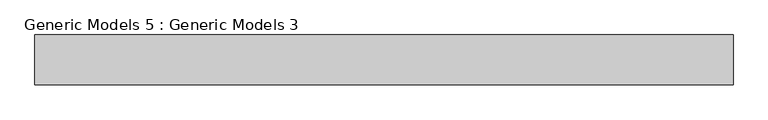
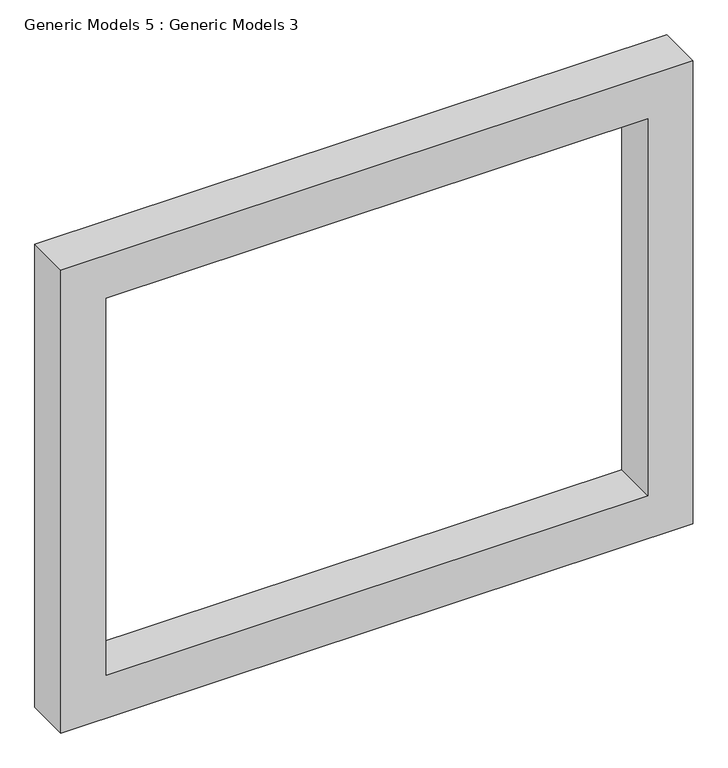
"""IFC4 building model written with IfcOpenShell, lengths in millimetres: proxy geometry, Generic Models 5 : Generic Models 3."""

from ifc_helpers import new_model, si_unit, frame, origin, place, context, project, spatial, polyline, outline, extrude, source, transform, mapped, element, save


def generic_models_5_generic_models_3_e9287e6f(model_context):
    return source(origin(), model_context, "Body", "SweptSolid", [
        extrude(outline(polyline([(5765.8, 4938.2671209), (5765.8, 2804.6671209), (4114.8, 2804.6671209), (4114.8, 4938.2671209), (5765.8, 4938.2671209)]), holes=[polyline([(5613.4, 4785.8671209), (4267.2, 4785.8671209), (4267.2, 2957.0671209), (5613.4, 2957.0671209), (5613.4, 4785.8671209)])]), frame((0.0, -2602.2776789, 0.0), z_axis=(0.0, 1.0, 0.0), x_axis=(0.0, 0.0, 1.0)), (0.0, 0.0, 1.0), 152.4),
    ])


if __name__ == "__main__":
    model = new_model("IFC4")
    model_context = context("Model", 3, world=origin())
    ifc_project = project(units=[si_unit("LENGTHUNIT", "METRE", prefix="MILLI")], contexts=[model_context])
    site = spatial("IfcSite", under=ifc_project)
    building = spatial("IfcBuilding", under=site)
    placement = place(None, origin())
    generic_models_5_generic_models_3_shape = generic_models_5_generic_models_3_e9287e6f(model_context)
    element("IfcBuildingElementProxy", 1, Name="Generic Models 5 : Generic Models 3", ObjectType="Generic Models 5 : Generic Models 3", at=placement, inside=building, context=model_context, shape_type="MappedRepresentation", body=[
        mapped(generic_models_5_generic_models_3_shape, transform((0.0, 0.0, 0.0), x_axis=(1.0, 0.0, 0.0), y_axis=(0.0, 1.0, 0.0), z_axis=(0.0, 0.0, 1.0))),
    ])
    save(model, "model.ifc")

# Revit data of these elements
# Element 1 (IfcBuildingElementProxy, "Generic Models 5 : Generic Models 3")
#   Materials on its faces: "WALNUT WOOD COLOUR 5\""
# Materials
#   "WALNUT WOOD COLOUR 5\"": class "Generic", colour RGB 120 120 120, transparency 0, Cost = 0
